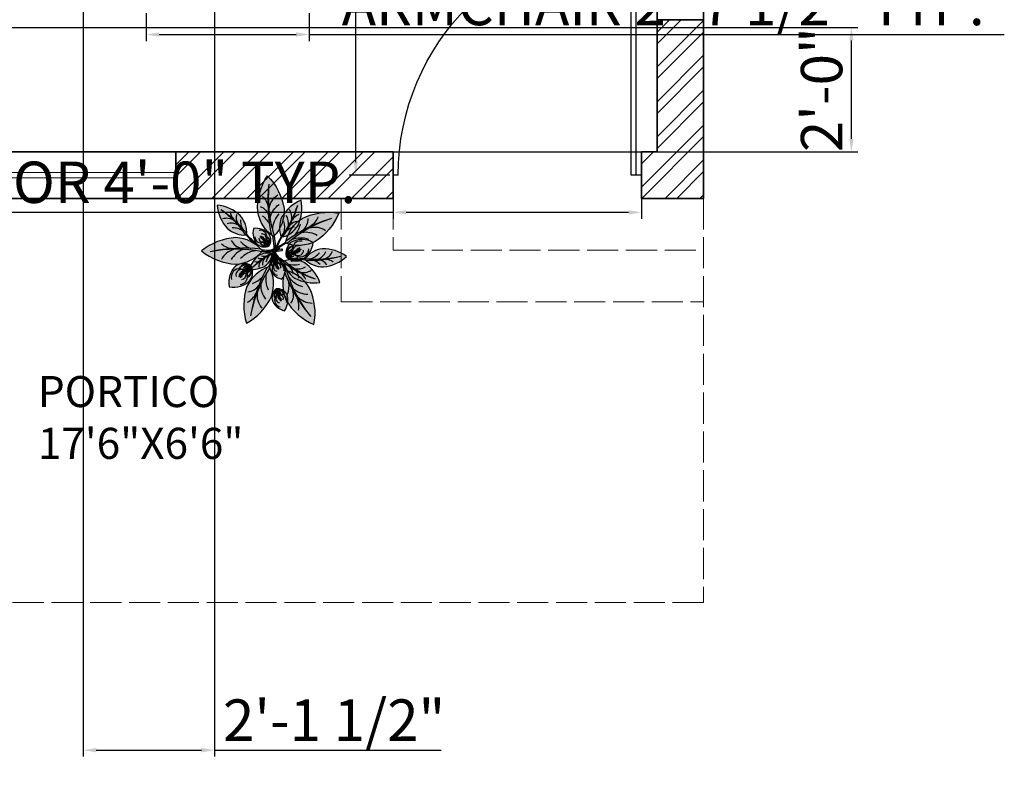
# Model space of a CAD drawing. Units: inches. Extents: x 3595 to 4516, y 2363 to 2965.
# Tile 8 of 12: x 4309 to 4499, y 2363 to 2512. Entities that reach past the tile are written whole.
import ezdxf

# ---------------------------------------------------------------- set-up
doc = ezdxf.new("R2010")
doc.units = ezdxf.units.IN
doc.linetypes.add('ACAD_ISO02W100', pattern=[15, 12, -3])
for name, color, linetype, lineweight in [('A-ANNO-DIMS', 2, 'Continuous', 18), ('A-AREA-IDEN', 7, 'Continuous', 18), ('A-DOOR', 4, 'Continuous', 25), ('A-FLOR-OTLN', 7, 'ACAD_ISO02W100', 18), ('A-FLOR-STRS-BYND', 7, 'ACAD_ISO02W100', 18), ('A-GLAZ', 4, 'Continuous', 18), ('A-WALL', 7, 'Continuous', 35), ('L-PLNT', 3, 'Continuous', 13)]:
    doc.layers.add(name, color=color, linetype=linetype, lineweight=lineweight)
doc.layers.add('A-WALL-PATT', color=251, linetype='Continuous', lineweight=13, true_color=0x636466)
doc.layers.add('MESA', color=7, linetype='Continuous')
doc.styles.get("Standard").update_dxf_attribs({"font": 'arial.ttf'})
doc.dimstyles.new('ISO-25', dxfattribs={"dimtxt": 8, "dimasz": 2.5, "dimexe": 1.25, "dimexo": 0.625, "dimtad": 1, "dimdec": 1, "dimlunit": 3, "dimtxsty": 'Standard', "dimcen": 2.5, "dimadec": 0, "dimazin": 0, "dimtfac": 1, "dimtdec": 1, "dimtmove": 0, "dimatfit": 3, "dimfxl": 1, "dimarcsym": 0})

# ---------------------------------------------------------------- blocks, each defined once
blk = doc.blocks.new('D')
for p, q in [((1, 0), (1, 46)), ((2, 0), (2, 46)), ((0, 0), (2, 0)), ((47, 0), (48, 0))]:
    blk.add_line(p, q)
at = {"ltscale": 0.5}
blk.add_arc((1, 0), 46, 0, 90, dxfattribs=at)
blk = doc.blocks.new('folha Ant')
at = {"layer": 'MESA', "ltscale": 0.8}
h = blk.add_hatch(color=256, dxfattribs=at)
h.dxf.hatch_style = 1
h.set_gradient(color1=(103, 159, 96), color2=(179, 207, 175), one_color=1, tint=0.75, name='INVCURVED')
h.paths.add_polyline_path([(0.2266, 0.0676, 0.199512), (0.0989, 0.0067, 0.09675), (0.3533, 0.0075, -0.086654), (0.1023, -0.0053, 0.192489), (0.2266, -0.0624, 0.158608), (0.3953, 0.0026, 0.158608)])
h = blk.add_hatch(color=256, dxfattribs=at)
h.dxf.hatch_style = 1
h.set_gradient(color1=(179, 116, 77), color2=(114, 74, 49), one_color=1, tint=0.32, name='CURVED')
h.paths.add_polyline_path([(0.05, -0.0003), (0.0485, 0.0057, 0.033108), (0, 0, 0.809082), (0.002, -0.006, -0.032777)])
h.paths.add_polyline_path([(0.0973, 0.0049, 0.033108), (0.0485, 0.0057), (0.05, -0.0003, -0.032777), (0.0983, -0.001), (0.0953, 0.0026)])
h = blk.add_hatch(color=256, dxfattribs=at)
h.dxf.hatch_style = 1
h.set_gradient(color1=(103, 159, 96), color2=(52, 80, 48), one_color=1, tint=0.25)
h.paths.add_polyline_path([(0.3533, 0.0075, -0.09675), (0.0989, 0.0067, 0.007527), (0.0953, 0.0026, 0.014292), (0.1023, -0.0053, 0.086654)])
blk.add_lwpolyline([(0.0983, -0.001), (0.0953, 0.0026), (0.0973, 0.0049, 0.066288), (0, 0, 0.809082), (0.002, -0.006, -0.065625)], format="xyb", close=True, dxfattribs=at)
for centre, radius, start, end in [((0.2359, -0.1164), 0.1842, 92.9121, 139.7695), ((0.211, -0.2242), 0.2922, 50.9055, 86.9554), ((0.2359, 0.1215), 0.1842, 220.2305, 267.0879), ((0.2242, 0.6583), 0.6635, 259.119, 281.2235), ((0.1912, 0.7199), 0.7306, 263.0097, 282.8199), ((0.1144, 0.1192), 0.1187, 277.6411, 318.482), ((0.1515, 0.1013), 0.1129, 290.5634, 330.4539), ((0.211, 0.2293), 0.2922, 273.0446, 309.0945), ((0.2123, 0.0879), 0.0955, 283.0013, 333.1911), ((0.1127, -0.1239), 0.1214, 41.7528, 70.1061), ((0.1853, -0.0821), 0.0727, 27.7376, 79.2347), ((0.2381, -0.0995), 0.0902, 48.8027, 88.011)]:
    blk.add_arc(centre, radius, start, end, dxfattribs=at)
blk = doc.blocks.new('folha A')
at = {"layer": 'MESA', "ltscale": 0.8}
h = blk.add_hatch(color=256, dxfattribs=at)
h.dxf.hatch_style = 1
h.set_gradient(color1=(237, 238, 238), one_color=1, tint=1)
h.paths.add_polyline_path([(0.15, 0, 0.256909), (0.0543, 0.05, 0.240303), (0.0028, 0.0075, -0.358381), (0.0489, 0.0306, 0.270233), (0, 0, -0.348977), (0.0363, 0.0149, 0.25095), (0.0039, 0, -0.245389), (0.0298, 0.008, 0.153246), (0.0082, 0, 0.15184), (0.0296, -0.008, 0.001374), (0.0298, -0.008, -0.245389), (0.0039, 0, 0.25095), (0.0363, -0.0149, -0.348977), (0, 0, 0.270233), (0.0489, -0.0306, -0.358381), (0.0028, -0.0075, 0.240303), (0.0543, -0.05, 0.256909)])
edge = h.paths.add_edge_path(flags=16)
edge.add_arc((0.0098, 0.0552), 0.0552, 269.916, 271.4154, ccw=False)
edge.add_arc((0.011, -0.0487), 0.0487, 89.8163, 91.5152, ccw=False)
edge.add_arc((0.0098, 0.0552), 0.0552, 271.4154, 288.9745)
edge.add_spline(control_points=[(0.0278, 0.003), (0.0281, 0.003), (0.03, 0.0028), (0.032, 0.0025), (0.0337, 0.0022)], knot_values=[0.247151, 0.247151, 0.247151, 0.247151, 0.247786, 0.253074, 0.253074, 0.253074, 0.253074], degree=3, periodic=0)
edge.add_spline(control_points=[(0.0337, 0.0022), (0.0349, 0.0021), (0.0361, 0.0019), (0.0372, 0.0017)], knot_values=[0.243636, 0.243636, 0.243636, 0.243636, 0.247151, 0.247151, 0.247151, 0.247151], degree=3, periodic=0)
edge.add_spline(control_points=[(0.0372, 0.0017), (0.0385, 0.0015), (0.0405, 0.0013), (0.0424, 0.0011), (0.0431, 0.0011)], knot_values=[0.23773, 0.23773, 0.23773, 0.23773, 0.241748, 0.243636, 0.243636, 0.243636, 0.243636], degree=3, periodic=0)
edge.add_spline(control_points=[(0.0431, 0.0011), (0.044, 0.001), (0.045, 0.001), (0.0459, 0.001)], knot_values=[0.234818, 0.234818, 0.234818, 0.234818, 0.23773, 0.23773, 0.23773, 0.23773], degree=3, periodic=0)
edge.add_spline(control_points=[(0.0459, 0.001), (0.0472, 0.0009), (0.0485, 0.0009), (0.0498, 0.0009)], knot_values=[0.230931, 0.230931, 0.230931, 0.230931, 0.234818, 0.234818, 0.234818, 0.234818], degree=3, periodic=0)
edge.add_spline(control_points=[(0.0498, 0.0009), (0.0513, 0.0009), (0.0528, 0.0009), (0.0543, 0.0009)], knot_values=[0.226471, 0.226471, 0.226471, 0.226471, 0.230931, 0.230931, 0.230931, 0.230931], degree=3, periodic=0)
edge.add_spline(control_points=[(0.0543, 0.0009), (0.0547, 0.0009), (0.0564, 0.001), (0.0581, 0.001), (0.0594, 0.0011)], knot_values=[0.221526, 0.221526, 0.221526, 0.221526, 0.222579, 0.226471, 0.226471, 0.226471, 0.226471], degree=3, periodic=0)
edge.add_spline(control_points=[(0.0594, 0.0011), (0.0609, 0.0012), (0.0623, 0.0014), (0.0637, 0.0017)], knot_values=[0.217168, 0.217168, 0.217168, 0.217168, 0.221526, 0.221526, 0.221526, 0.221526], degree=3, periodic=0)
edge.add_spline(control_points=[(0.0637, 0.0017), (0.0648, 0.002), (0.066, 0.0024), (0.0672, 0.0029), (0.0674, 0.003)], knot_values=[0.213164, 0.213164, 0.213164, 0.213164, 0.216463, 0.217168, 0.217168, 0.217168, 0.217168], degree=3, periodic=0)
edge.add_spline(control_points=[(0.0674, 0.003), (0.0685, 0.0035), (0.07, 0.0044), (0.0718, 0.0051), (0.0724, 0.0052)], knot_values=[0.207777, 0.207777, 0.207777, 0.207777, 0.211372, 0.213164, 0.213164, 0.213164, 0.213164], degree=3, periodic=0)
edge.add_spline(control_points=[(0.0724, 0.0052), (0.0729, 0.0053), (0.0744, 0.0054), (0.0757, 0.0044), (0.0762, 0.0036)], knot_values=[0.203445, 0.203445, 0.203445, 0.203445, 0.204995, 0.207777, 0.207777, 0.207777, 0.207777], degree=3, periodic=0)
edge.add_spline(control_points=[(0.0762, 0.0036), (0.0763, 0.0036), (0.0768, 0.0026), (0.0767, 0.0012), (0.0763, 0), (0.0763, -0.0001)], knot_values=[0.199694, 0.199694, 0.199694, 0.199694, 0.199863, 0.203137, 0.203445, 0.203445, 0.203445, 0.203445], degree=3, periodic=0)
edge.add_spline(control_points=[(0.0763, -0.0001), (0.0761, -0.0008), (0.0757, -0.0017), (0.075, -0.0024), (0.0748, -0.0026)], knot_values=[0.196756, 0.196756, 0.196756, 0.196756, 0.198903, 0.199694, 0.199694, 0.199694, 0.199694], degree=3, periodic=0)
edge.add_spline(control_points=[(0.0748, -0.0026), (0.0743, -0.0031), (0.0734, -0.0037), (0.0725, -0.0042), (0.0722, -0.0043)], knot_values=[0.193643, 0.193643, 0.193643, 0.193643, 0.195869, 0.196756, 0.196756, 0.196756, 0.196756], degree=3, periodic=0)
edge.add_spline(control_points=[(0.0722, -0.0043), (0.0708, -0.0049), (0.0694, -0.0052), (0.0678, -0.0054)], knot_values=[0.189135, 0.189135, 0.189135, 0.189135, 0.193643, 0.193643, 0.193643, 0.193643], degree=3, periodic=0)
edge.add_spline(control_points=[(0.0678, -0.0054), (0.0677, -0.0054), (0.0667, -0.0056), (0.0657, -0.0057), (0.0648, -0.0058)], knot_values=[0.186092, 0.186092, 0.186092, 0.186092, 0.186502, 0.189135, 0.189135, 0.189135, 0.189135], degree=3, periodic=0)
edge.add_spline(control_points=[(0.0648, -0.0058), (0.0635, -0.0059), (0.0621, -0.006), (0.0608, -0.0061)], knot_values=[0.182083, 0.182083, 0.182083, 0.182083, 0.186092, 0.186092, 0.186092, 0.186092], degree=3, periodic=0)
edge.add_spline(control_points=[(0.0608, -0.0061), (0.0596, -0.0062), (0.0584, -0.0062), (0.0571, -0.0062)], knot_values=[0.178391, 0.178391, 0.178391, 0.178391, 0.182083, 0.182083, 0.182083, 0.182083], degree=3, periodic=0)
edge.add_spline(control_points=[(0.0571, -0.0062), (0.0568, -0.0062), (0.0555, -0.0063), (0.0543, -0.0063), (0.0534, -0.0063)], knot_values=[0.17468, 0.17468, 0.17468, 0.17468, 0.175797, 0.178391, 0.178391, 0.178391, 0.178391], degree=3, periodic=0)
edge.add_spline(control_points=[(0.0534, -0.0063), (0.0525, -0.0063), (0.0516, -0.0063), (0.0506, -0.0063)], knot_values=[0.171864, 0.171864, 0.171864, 0.171864, 0.17468, 0.17468, 0.17468, 0.17468], degree=3, periodic=0)
edge.add_spline(control_points=[(0.0506, -0.0063), (0.0494, -0.0063), (0.0482, -0.0063), (0.047, -0.0062)], knot_values=[0.16826, 0.16826, 0.16826, 0.16826, 0.171864, 0.171864, 0.171864, 0.171864], degree=3, periodic=0)
edge.add_spline(control_points=[(0.047, -0.0062), (0.0453, -0.0061), (0.0434, -0.006), (0.0414, -0.0057), (0.0411, -0.0057)], knot_values=[0.162342, 0.162342, 0.162342, 0.162342, 0.167388, 0.16826, 0.16826, 0.16826, 0.16826], degree=3, periodic=0)
edge.add_spline(control_points=[(0.0411, -0.0057), (0.0399, -0.0055), (0.0386, -0.0053), (0.0374, -0.005)], knot_values=[0.158654, 0.158654, 0.158654, 0.158654, 0.162342, 0.162342, 0.162342, 0.162342], degree=3, periodic=0)
edge.add_spline(control_points=[(0.0374, -0.005), (0.0365, -0.0049), (0.0357, -0.0047), (0.0348, -0.0045)], knot_values=[0.156033, 0.156033, 0.156033, 0.156033, 0.158654, 0.158654, 0.158654, 0.158654], degree=3, periodic=0)
edge.add_spline(control_points=[(0.0348, -0.0045), (0.0335, -0.0043), (0.0317, -0.004), (0.03, -0.0037), (0.0295, -0.0036)], knot_values=[0.15048, 0.15048, 0.15048, 0.15048, 0.154549, 0.156033, 0.156033, 0.156033, 0.156033], degree=3, periodic=0)
edge.add_arc((0.011, -0.0487), 0.0487, 67.7054, 89.8163)
h = blk.add_hatch(color=256, dxfattribs=at)
h.dxf.hatch_style = 1
h.set_gradient(color1=(117, 211, 105), one_color=1, tint=1)
h.paths.add_polyline_path([(0.0489, 0.0306, 0.358381), (0.0028, 0.0075, 0.02724), (0, 0, -0.270233)])
h.paths.add_polyline_path([(0.0039, 0, -0.25095), (0.0363, 0.0149, 0.348977), (0, 0, 0.348977), (0.0363, -0.0149, -0.25095)])
h.paths.add_polyline_path([(0.0298, 0.008, 0.245389), (0.0039, 0, 0.245389), (0.0298, -0.008, -0.153246), (0.0082, 0, -0.153246)], flags=17)
h.paths.add_polyline_path([(0, 0, 0.02724), (0.0028, -0.0075, 0.358381), (0.0489, -0.0306, -0.270233)])
h = blk.add_hatch(color=256, dxfattribs=at)
h.dxf.hatch_style = 1
h.set_gradient(color1=(68, 182, 53), color2=(121, 213, 109), one_color=1, tint=0.63, name='CYLINDER')
edge = h.paths.add_edge_path()
edge.add_spline(control_points=[(0.0722, -0.0043), (0.0725, -0.0042), (0.0734, -0.0037), (0.0743, -0.0031), (0.0748, -0.0026)], knot_values=[0.193643, 0.193643, 0.193643, 0.193643, 0.194531, 0.196756, 0.196756, 0.196756, 0.196756], degree=3, periodic=0)
edge.add_spline(control_points=[(0.0748, -0.0026), (0.075, -0.0024), (0.0757, -0.0017), (0.0761, -0.0008), (0.0763, -0.0001)], knot_values=[0.196756, 0.196756, 0.196756, 0.196756, 0.197548, 0.199694, 0.199694, 0.199694, 0.199694], degree=3, periodic=0)
edge.add_spline(control_points=[(0.0763, -0.0001), (0.0763, 0), (0.0767, 0.0012), (0.0768, 0.0026), (0.0763, 0.0036), (0.0762, 0.0036)], knot_values=[0.199694, 0.199694, 0.199694, 0.199694, 0.200002, 0.203276, 0.203445, 0.203445, 0.203445, 0.203445], degree=3, periodic=0)
edge.add_spline(control_points=[(0.0762, 0.0036), (0.0757, 0.0044), (0.0744, 0.0054), (0.0729, 0.0053), (0.0724, 0.0052)], knot_values=[0.203445, 0.203445, 0.203445, 0.203445, 0.206228, 0.207777, 0.207777, 0.207777, 0.207777], degree=3, periodic=0)
edge.add_spline(control_points=[(0.0724, 0.0052), (0.0718, 0.0051), (0.07, 0.0044), (0.0685, 0.0035), (0.0674, 0.003)], knot_values=[0.207777, 0.207777, 0.207777, 0.207777, 0.20957, 0.213164, 0.213164, 0.213164, 0.213164], degree=3, periodic=0)
edge.add_spline(control_points=[(0.0674, 0.003), (0.0672, 0.0029), (0.066, 0.0024), (0.0648, 0.002), (0.0637, 0.0017)], knot_values=[0.213164, 0.213164, 0.213164, 0.213164, 0.213868, 0.217168, 0.217168, 0.217168, 0.217168], degree=3, periodic=0)
edge.add_spline(control_points=[(0.0637, 0.0017), (0.0623, 0.0014), (0.0609, 0.0012), (0.0594, 0.0011)], knot_values=[0.217168, 0.217168, 0.217168, 0.217168, 0.221526, 0.221526, 0.221526, 0.221526], degree=3, periodic=0)
edge.add_spline(control_points=[(0.0594, 0.0011), (0.0581, 0.001), (0.0564, 0.001), (0.0547, 0.0009), (0.0543, 0.0009)], knot_values=[0.221526, 0.221526, 0.221526, 0.221526, 0.225418, 0.226471, 0.226471, 0.226471, 0.226471], degree=3, periodic=0)
edge.add_spline(control_points=[(0.0543, 0.0009), (0.0528, 0.0009), (0.0513, 0.0009), (0.0498, 0.0009)], knot_values=[0.226471, 0.226471, 0.226471, 0.226471, 0.230931, 0.230931, 0.230931, 0.230931], degree=3, periodic=0)
edge.add_spline(control_points=[(0.0498, 0.0009), (0.0485, 0.0009), (0.0472, 0.0009), (0.0459, 0.001)], knot_values=[0.230931, 0.230931, 0.230931, 0.230931, 0.234818, 0.234818, 0.234818, 0.234818], degree=3, periodic=0)
edge.add_spline(control_points=[(0.0459, 0.001), (0.045, 0.001), (0.044, 0.001), (0.0431, 0.0011)], knot_values=[0.234818, 0.234818, 0.234818, 0.234818, 0.23773, 0.23773, 0.23773, 0.23773], degree=3, periodic=0)
edge.add_spline(control_points=[(0.0431, 0.0011), (0.0424, 0.0011), (0.0405, 0.0013), (0.0385, 0.0015), (0.0372, 0.0017)], knot_values=[0.23773, 0.23773, 0.23773, 0.23773, 0.239619, 0.243636, 0.243636, 0.243636, 0.243636], degree=3, periodic=0)
edge.add_spline(control_points=[(0.0372, 0.0017), (0.0361, 0.0019), (0.0349, 0.0021), (0.0337, 0.0022)], knot_values=[0.243636, 0.243636, 0.243636, 0.243636, 0.247151, 0.247151, 0.247151, 0.247151], degree=3, periodic=0)
edge.add_spline(control_points=[(0.0337, 0.0022), (0.032, 0.0025), (0.03, 0.0028), (0.0281, 0.003), (0.0278, 0.003)], knot_values=[0.247151, 0.247151, 0.247151, 0.247151, 0.25244, 0.253074, 0.253074, 0.253074, 0.253074], degree=3, periodic=0)
edge.add_arc((0.011, 0.0487), 0.0487, 271.5152, 290.2274, ccw=False)
edge.add_arc((0.011, -0.0487), 0.0487, 67.7054, 88.4848, ccw=False)
edge.add_spline(control_points=[(0.0295, -0.0036), (0.03, -0.0037), (0.0317, -0.004), (0.0335, -0.0043), (0.0348, -0.0045)], knot_values=[0.15048, 0.15048, 0.15048, 0.15048, 0.151964, 0.156033, 0.156033, 0.156033, 0.156033], degree=3, periodic=0)
edge.add_spline(control_points=[(0.0348, -0.0045), (0.0357, -0.0047), (0.0365, -0.0049), (0.0374, -0.005)], knot_values=[0.156033, 0.156033, 0.156033, 0.156033, 0.158654, 0.158654, 0.158654, 0.158654], degree=3, periodic=0)
edge.add_spline(control_points=[(0.0374, -0.005), (0.0386, -0.0053), (0.0399, -0.0055), (0.0411, -0.0057)], knot_values=[0.158654, 0.158654, 0.158654, 0.158654, 0.162342, 0.162342, 0.162342, 0.162342], degree=3, periodic=0)
edge.add_spline(control_points=[(0.0411, -0.0057), (0.0414, -0.0057), (0.0434, -0.006), (0.0453, -0.0061), (0.047, -0.0062)], knot_values=[0.162342, 0.162342, 0.162342, 0.162342, 0.163214, 0.16826, 0.16826, 0.16826, 0.16826], degree=3, periodic=0)
edge.add_spline(control_points=[(0.047, -0.0062), (0.0482, -0.0063), (0.0494, -0.0063), (0.0506, -0.0063)], knot_values=[0.16826, 0.16826, 0.16826, 0.16826, 0.171864, 0.171864, 0.171864, 0.171864], degree=3, periodic=0)
edge.add_spline(control_points=[(0.0506, -0.0063), (0.0516, -0.0063), (0.0525, -0.0063), (0.0534, -0.0063)], knot_values=[0.171864, 0.171864, 0.171864, 0.171864, 0.17468, 0.17468, 0.17468, 0.17468], degree=3, periodic=0)
edge.add_spline(control_points=[(0.0534, -0.0063), (0.0543, -0.0063), (0.0555, -0.0063), (0.0568, -0.0062), (0.0571, -0.0062)], knot_values=[0.17468, 0.17468, 0.17468, 0.17468, 0.177274, 0.178391, 0.178391, 0.178391, 0.178391], degree=3, periodic=0)
edge.add_spline(control_points=[(0.0571, -0.0062), (0.0584, -0.0062), (0.0596, -0.0062), (0.0608, -0.0061)], knot_values=[0.178391, 0.178391, 0.178391, 0.178391, 0.182083, 0.182083, 0.182083, 0.182083], degree=3, periodic=0)
edge.add_spline(control_points=[(0.0608, -0.0061), (0.0621, -0.006), (0.0635, -0.0059), (0.0648, -0.0058)], knot_values=[0.182083, 0.182083, 0.182083, 0.182083, 0.186092, 0.186092, 0.186092, 0.186092], degree=3, periodic=0)
edge.add_spline(control_points=[(0.0648, -0.0058), (0.0657, -0.0057), (0.0667, -0.0056), (0.0677, -0.0054), (0.0678, -0.0054)], knot_values=[0.186092, 0.186092, 0.186092, 0.186092, 0.188726, 0.189135, 0.189135, 0.189135, 0.189135], degree=3, periodic=0)
edge.add_spline(control_points=[(0.0678, -0.0054), (0.0694, -0.0052), (0.0708, -0.0049), (0.0722, -0.0043)], knot_values=[0.189135, 0.189135, 0.189135, 0.189135, 0.193643, 0.193643, 0.193643, 0.193643], degree=3, periodic=0)
for p, q in [((0.0299, -0.0008), (0.0236, 0.0003)), ((0.0324, 0.0004), (0.0358, 0.0051)), ((0.0367, 0.001), (0.0414, 0.0073)), ((0.0435, -0.0027), (0.0427, 0.0041)), ((0.0455, -0.0007), (0.0466, 0.0032)), ((0.0507, -0.0021), (0.0477, 0.0086)), ((0.0545, -0.0006), (0.0538, 0.005)), ((0.0604, -0.0013), (0.0571, 0.0065)), ((0.0637, -0.0003), (0.0638, 0.0057)), ((0.0674, 0.0003), (0.0674, 0.0088)), ((0.071, 0.0011), (0.0736, 0.0087)), ((0.0744, 0.0005), (0.0836, -0.0024)), ((0.0745, 0.0023), (0.0809, 0.0072)), ((0.0331, -0.0017), (0.0356, -0.0058)), ((0.0359, -0.0021), (0.0384, -0.0071)), ((0.04, -0.0018), (0.0423, -0.0098)), ((0.0474, -0.0047), (0.0459, -0.0105)), ((0.0512, -0.005), (0.0493, -0.009)), ((0.0546, -0.0037), (0.0519, -0.0097)), ((0.0571, -0.0045), (0.0573, -0.0126)), ((0.0629, -0.0036), (0.0579, -0.0096)), ((0.0649, -0.0044), (0.0646, -0.0097)), ((0.0679, -0.003), (0.0676, -0.0121)), ((0.0718, -0.0029), (0.0733, -0.0082)), ((0.0731, -0.0013), (0.0781, -0.005))]:
    blk.add_line(p, q, dxfattribs=at)
for centre, radius, start, end in [((0.0702, -0.0218), 0.0735, 102.4876, 162.7777), ((0.0567, -0.062), 0.112, 33.595, 91.2278), ((0.0507, -0.0267), 0.0573, 91.7664, 152.2545), ((0.0275, -0.0154), 0.0315, 73.8983, 150.8496), ((0.0399, -0.009), 0.0406, 77.1426, 158.365), ((0.034, -0.0228), 0.0378, 86.5852, 142.9351), ((0.0245, -0.0208), 0.0293, 79.5747, 134.724), ((0.0317, -0.0305), 0.0385, 92.8652, 127.7155), ((0.0067, 0.0482), 0.0483, 273.5313, 328.711), ((0.0098, 0.0552), 0.0552, 269.916, 311.5613), ((0.011, -0.0487), 0.0487, 43.3703, 91.5152), ((0.0655, -0.0023), 0.025, 51.9712, 139.685), ((0.0788, 0.0012), 0.0378, 48.9446, 144.5333), ((0.0507, 0.0267), 0.0573, 207.7455, 268.2336), ((0.0275, 0.0154), 0.0315, 209.1504, 286.1017), ((0.0702, 0.0218), 0.0735, 197.2223, 257.5124), ((0.0399, 0.009), 0.0406, 201.635, 282.8574), ((0.034, 0.0228), 0.0378, 217.0649, 273.4148), ((0.0245, 0.0208), 0.0293, 225.276, 280.4253), ((0.0317, 0.0305), 0.0385, 232.2845, 267.1348), ((0.0067, -0.0482), 0.0483, 31.289, 86.4687), ((0.0676, -0.0011), 0.0254, 213.677, 332.8415), ((0.0804, 0.0017), 0.0409, 217.4348, 331.7322), ((0.0567, 0.062), 0.112, 268.7722, 326.405)]:
    blk.add_arc(centre, radius, start, end, dxfattribs=at)
blk.add_open_spline([(0.0295, -0.0036), (0.03, -0.0037), (0.0339, -0.0043), (0.0429, -0.0064), (0.0552, -0.0064), (0.0655, -0.0059), (0.0723, -0.0047), (0.0754, -0.0023), (0.0766, 0.0004), (0.0769, 0.0036), (0.0738, 0.0058), (0.0702, 0.0046), (0.0648, 0.0013), (0.0544, 0.0009), (0.0416, 0.0008), (0.0325, 0.0025), (0.0281, 0.003), (0.0278, 0.003)], degree=3, knots=[0.1504802, 0.1504802, 0.1504802, 0.1504802, 0.1519644, 0.163214, 0.177274, 0.1887256, 0.1945307, 0.1975476, 0.2000024, 0.2032763, 0.2062279, 0.2095699, 0.2138685, 0.2254176, 0.2396186, 0.2524399, 0.2530743, 0.2530743, 0.2530743, 0.2530743], dxfattribs=at)
blk = doc.blocks.new('Anturio Completa')
at = {"layer": 'MESA', "xscale": -1}
for p, rotation in [((0.0382, -0.3934), 275.9103487005753), ((0.0047, -0.3743), 209.3422747969654)]:
    blk.add_blockref('folha Ant', p, dxfattribs=dict(at, rotation=rotation))
at = {"layer": 'MESA'}
for name, p, xscale, yscale, zscale, rotation in [('folha Ant', (-0.0545, -0.3355), 0.6875195991113106, 0.6875195991113106, 0.6875195991113106, 134.6123703789177), ('folha Ant', (0.0396, -0.3604), 0.6875195991112988, 0.6875195991112988, 0.6875195991112988, 62.02852832027476), ('folha A', (0.0091, -0.3436), 0.7678141644548924, 0.7678141644548924, 0.7678141644548924, 132.2423739965673), ('folha Ant', (0.06, -0.3566), 0.4588451896756128, 0.4588451896756128, 0.4588451896756128, 214.0760858842101), ('folha A', (0.0322, -0.3992), 0.7678141644548587, 0.7678141644548587, 0.7678141644548587, 290.0444626994612), ('folha Ant', (0.0225, -0.3869), 0.6875195991113232, 0.6875195991113232, 0.6875195991113232, 329.7037252995857), ('folha Ant', (0.1178, -0.4144), 0.6875195991112375, 0.6875195991112375, 0.6875195991112375, 3.732606609119443), ('folha A', (0.0446, -0.5537), 0.7678141644548587, 0.7678141644548587, 0.7678141644548587, 290.0444626994612)]:
    blk.add_blockref(name, p, dxfattribs=dict(at, xscale=xscale, yscale=yscale, zscale=zscale, rotation=rotation))
for name, p, rotation in [('folha A', (0.0917, -0.3951), 27.20904127110871), ('folha Ant', (0.0722, -0.3656), 180), ('folha Ant', (0.0428, -0.3558), 248.0349850699403), ('folha Ant', (0.0423, -0.3813), 297.7195320534174), ('folha A', (-0.0806, -0.4387), 224.8255080541778)]:
    blk.add_blockref(name, p, dxfattribs=dict(at, rotation=rotation))
blk = doc.blocks.new('WIN-GLAZING-66IN')
for p, q in [((0, 1), (66, 1)), ((0, 0), (66, 0))]:
    blk.add_line(p, q)
blk = doc.blocks.new('PORTICO-ENTRY-STEPS')
at = {"ltscale": 0.5}
for p, q in [((0, 20), (0, 0)), ((10, 20), (10, 10)), ((10, 10), (70, 10)), ((0, 0), (70, 0))]:
    blk.add_line(p, q, dxfattribs=at)
blk = doc.blocks.new('*D113')
at = {"layer": 'A-ANNO-DIMS', "color": 0, "lineweight": -2, "transparency": 16777216}
for p, q in [((4381.24, 2480.92), (4381.24, 2473.09)), ((4429.24, 2480.92), (4429.24, 2473.09)), ((4381.24, 2474.34), (4251.53, 2474.34)), ((4426.74, 2474.34), (4383.74, 2474.34))]:
    blk.add_line(p, q, dxfattribs=at)
at = {"layer": 'A-ANNO-DIMS', "color": 0, "transparency": 16777216}
for points in [[(4383.74, 2474.76), (4383.74, 2473.93), (4381.24, 2474.34)], [(4426.74, 2474.76), (4426.74, 2473.93), (4429.24, 2474.34)]]:
    blk.add_solid(points, dxfattribs=at)
at = {"layer": 'Defpoints', "color": 0, "transparency": 16777216}
for p in [(4381.24, 2481.54), (4429.24, 2481.54), (4381.24, 2474.34)]:
    blk.add_point(p, dxfattribs=at)
at = {"layer": 'A-ANNO-DIMS', "color": 0, "transparency": 16777216, "insert": (4315.14, 2479.11), "char_height": 8, "attachment_point": 5}
blk.add_mtext('ENTRY DOOR 4\'-0" TYP.', dxfattribs=at)
blk = doc.blocks.new('*D114')
at = {"layer": 'A-ANNO-DIMS', "color": 0, "lineweight": -2, "transparency": 16777216}
for p, q in [((4374.04, 2527.54), (4374.04, 2586.27)), ((4380.62, 2527.54), (4372.79, 2527.54)), ((4374.04, 2484.04), (4374.04, 2525.04)), ((4380.62, 2481.54), (4372.79, 2481.54))]:
    blk.add_line(p, q, dxfattribs=at)
at = {"layer": 'A-ANNO-DIMS', "color": 0, "transparency": 16777216}
for points in [[(4373.63, 2525.04), (4374.46, 2525.04), (4374.04, 2527.54)], [(4373.63, 2484.04), (4374.46, 2484.04), (4374.04, 2481.54)]]:
    blk.add_solid(points, dxfattribs=at)
at = {"layer": 'Defpoints', "color": 0, "transparency": 16777216}
for p in [(4374.04, 2527.54), (4381.24, 2527.54), (4381.24, 2481.54)]:
    blk.add_point(p, dxfattribs=at)
at = {"layer": 'A-ANNO-DIMS', "color": 0, "transparency": 16777216, "insert": (4369.33, 2558.16), "char_height": 8, "attachment_point": 5, "rotation": 90}
blk.add_mtext('3\'-10" TYP.', dxfattribs=at)
blk = doc.blocks.new('*D139')
at = {"layer": 'A-ANNO-DIMS', "color": 0, "lineweight": -2, "transparency": 16777216}
for p, q in [((4333.52, 2512.78), (4333.52, 2507.43)), ((4365.01, 2512.78), (4365.01, 2507.43)), ((4336.02, 2508.68), (4362.51, 2508.68)), ((4365.01, 2508.68), (4499.34, 2508.68))]:
    blk.add_line(p, q, dxfattribs=at)
at = {"layer": 'A-ANNO-DIMS', "color": 0, "transparency": 16777216}
for points in [[(4336.02, 2509.1), (4336.02, 2508.27), (4333.52, 2508.68)], [(4362.51, 2509.1), (4362.51, 2508.27), (4365.01, 2508.68)]]:
    blk.add_solid(points, dxfattribs=at)
at = {"layer": 'Defpoints', "color": 0, "transparency": 16777216}
for p in [(4333.52, 2513.41), (4365.01, 2513.41), (4365.01, 2508.68)]:
    blk.add_point(p, dxfattribs=at)
at = {"layer": 'A-ANNO-DIMS', "color": 0, "transparency": 16777216, "insert": (4433.43, 2513.44), "char_height": 8, "attachment_point": 5}
blk.add_mtext('ARMCHAIR 2\'-7 1/2" TYP.', dxfattribs=at)
blk = doc.blocks.new('*D160')
at = {"layer": 'A-ANNO-DIMS', "color": 0, "lineweight": -2, "transparency": 16777216}
for p, q in [((4114.87, 2510.04), (4471.04, 2510.04)), ((4469.79, 2488.54), (4469.79, 2507.54)), ((4090.87, 2486.04), (4471.04, 2486.04))]:
    blk.add_line(p, q, dxfattribs=at)
at = {"layer": 'A-ANNO-DIMS', "color": 0, "transparency": 16777216}
for points in [[(4469.38, 2507.54), (4470.21, 2507.54), (4469.79, 2510.04)], [(4469.38, 2488.54), (4470.21, 2488.54), (4469.79, 2486.04)]]:
    blk.add_solid(points, dxfattribs=at)
at = {"layer": 'Defpoints', "color": 0, "transparency": 16777216}
for p in [(4114.24, 2510.04), (4469.79, 2510.04), (4090.24, 2486.04)]:
    blk.add_point(p, dxfattribs=at)
at = {"layer": 'A-ANNO-DIMS', "color": 0, "transparency": 16777216, "insert": (4465.08, 2498.04), "char_height": 8, "attachment_point": 5, "rotation": 90}
blk.add_mtext('2\'-0"', dxfattribs=at)
blk = doc.blocks.new('*D161')
at = {"layer": 'A-ANNO-DIMS', "color": 0, "lineweight": -2, "transparency": 16777216}
for p, q in [((4321.38, 2565.12), (4321.38, 2369.24)), ((4346.72, 2565.12), (4346.72, 2369.24)), ((4323.88, 2370.49), (4344.22, 2370.49)), ((4346.72, 2370.49), (4390.51, 2370.49))]:
    blk.add_line(p, q, dxfattribs=at)
at = {"layer": 'A-ANNO-DIMS', "color": 0, "transparency": 16777216}
for points in [[(4323.88, 2370.91), (4323.88, 2370.08), (4321.38, 2370.49)], [(4344.22, 2370.91), (4344.22, 2370.08), (4346.72, 2370.49)]]:
    blk.add_solid(points, dxfattribs=at)
at = {"layer": 'Defpoints', "color": 0, "transparency": 16777216}
for p in [(4321.38, 2565.75), (4346.72, 2565.75), (4346.72, 2370.49)]:
    blk.add_point(p, dxfattribs=at)
at = {"layer": 'A-ANNO-DIMS', "color": 0, "transparency": 16777216, "insert": (4369.86, 2375.26), "char_height": 8, "attachment_point": 5}
blk.add_mtext('2\'-1 1/2"', dxfattribs=at)

msp = doc.modelspace()

# ---------------------------------------------------------------- hatches: boundary and pattern name
at = {"layer": 'A-WALL-PATT'}
h = msp.add_hatch(dxfattribs=at)
h.set_pattern_fill('ANSI32', color=256, scale=0.5)
h.set_pattern_definition([(45, (441.351, 0), (-3.367596, 3.367596), []), (45, (443.596, 0), (-3.367596, 3.367596), [])])
h.paths.add_polyline_path([(4081.24, 2756.04), (4090.24, 2756.04), (4090.24, 2894.04), (4168.24, 2894.04), (4168.24, 2903.04), (4081.24, 2903.04)])
h.paths.add_polyline_path([(4216.24, 2903.04), (4216.24, 2894.04), (4222.24, 2894.04), (4222.24, 2792.04), (4231.24, 2792.04), (4231.24, 2894.04), (4241.74, 2894.04), (4241.74, 2903.04)])
h.paths.add_polyline_path([(4324.24, 2894.04), (4324.24, 2903.04), (4277.74, 2903.04), (4277.74, 2894.04), (4288.24, 2894.04), (4288.24, 2798.04), (4261.24, 2798.04), (4261.24, 2792.04), (4288.24, 2792.04), (4288.24, 2756.04), (4222.24, 2756.04), (4222.24, 2702.04), (4219.24, 2702.04), (4219.24, 2693.04), (4241.74, 2693.04), (4241.74, 2702.04), (4231.24, 2702.04), (4231.24, 2750.04), (4288.24, 2750.04), (4288.24, 2702.04), (4277.74, 2702.04), (4277.74, 2693.04), (4393.24, 2693.04), (4393.24, 2702.04), (4294.24, 2702.04), (4294.24, 2840.04), (4396.24, 2840.04), (4396.24, 2846.04), (4294.24, 2846.04), (4294.24, 2894.04)])
h.paths.add_polyline_path([(4390.24, 2894.04), (4390.24, 2876.04), (4396.24, 2876.04), (4396.24, 2894.04), (4432.24, 2894.04), (4432.24, 2795.04), (4441.24, 2795.04), (4441.24, 2903.04), (4360.24, 2903.04), (4360.24, 2894.04)])
h.paths.add_polyline_path([(4090.24, 2693.04), (4183.24, 2693.04), (4183.24, 2702.04), (4090.24, 2702.04), (4090.24, 2708.04), (4081.24, 2708.04), (4081.24, 2673.54), (4090.24, 2673.54)])
h.paths.add_polyline_path([(4090.24, 2600.04), (4183.24, 2600.04), (4183.24, 2606.04), (4090.24, 2606.04), (4090.24, 2625.54), (4081.24, 2625.54), (4081.24, 2561.04), (4090.24, 2561.04)])
h.paths.add_polyline_path([(4081.24, 2399.04), (4231.24, 2399.04), (4231.24, 2405.04), (4090.24, 2405.04), (4090.24, 2477.04), (4180.24, 2477.04), (4180.24, 2486.04), (4090.24, 2486.04), (4090.24, 2525.04), (4081.24, 2525.04)])
h.paths.add_polyline_path([(4231.24, 2486.04), (4231.24, 2606.04), (4219.24, 2606.04), (4219.24, 2600.04), (4222.24, 2600.04), (4222.24, 2486.04), (4216.24, 2486.04), (4216.24, 2477.04), (4273.24, 2477.04), (4273.24, 2486.04)])
h.paths.add_polyline_path([(4339.24, 2486.04), (4339.24, 2477.04), (4381.24, 2477.04), (4381.24, 2486.04)])
h.paths.add_polyline_path([(4432.24, 2486.04), (4429.24, 2486.04), (4429.24, 2477.04), (4441.24, 2477.04), (4441.24, 2511.54), (4432.24, 2511.54)])
h.paths.add_polyline_path([(4432.24, 2571.54), (4441.24, 2571.54), (4441.24, 2607.54), (4432.24, 2607.54)])
h.paths.add_polyline_path([(4441.24, 2747.04), (4432.24, 2747.04), (4432.24, 2702.04), (4429.24, 2702.04), (4429.24, 2693.04), (4432.24, 2693.04), (4432.24, 2667.54), (4441.24, 2667.54)])

# ---------------------------------------------------------------- linework, layer by layer
at = {"layer": 'A-FLOR-OTLN', "ltscale": 0.5}
for p, q in [((4441.24, 2477.04), (4441.24, 2399.04)), ((4441.24, 2399.04), (4231.24, 2399.04))]:
    msp.add_line(p, q, dxfattribs=at)
at = {"layer": 'A-WALL'}
for p, q in [((4432.24, 2693.04), (4432.24, 2486.04)), ((4441.24, 2511.54), (4432.24, 2511.54)), ((4231.24, 2486.04), (4381.24, 2486.04)), ((4339.24, 2486.04), (4339.24, 2477.04)), ((4381.24, 2486.04), (4381.24, 2477.04)), ((4429.24, 2486.04), (4432.24, 2486.04)), ((4429.24, 2486.04), (4429.24, 2477.04)), ((4090.24, 2477.04), (4381.24, 2477.04)), ((4429.24, 2477.04), (4441.24, 2477.04))]:
    msp.add_line(p, q, dxfattribs=at)
msp.add_lwpolyline([(4231.24, 2399.04), (4081.24, 2399.04), (4081.24, 2903.04), (4441.24, 2903.04), (4441.24, 2477.04)], dxfattribs=at)

# ---------------------------------------------------------------- block references
at = {"layer": 'A-DOOR', "xscale": -1}
msp.add_blockref('D', (4429.24, 2481.54), dxfattribs=at)
at = {"layer": 'A-FLOR-STRS-BYND'}
msp.add_blockref('PORTICO-ENTRY-STEPS', (4371.24, 2457.04), dxfattribs=at)
at = {"layer": 'A-GLAZ'}
msp.add_blockref('WIN-GLAZING-66IN', (4273.24, 2481.04), dxfattribs=at)
at = {"layer": 'L-PLNT', "xscale": 39.3701, "yscale": 39.3701, "zscale": 39.3701}
msp.add_blockref('Anturio Completa', (4356.95, 2481.4), dxfattribs=at)

# ---------------------------------------------------------------- texts
at = {"layer": 'A-AREA-IDEN', "insert": (4312.61, 2442.74), "char_height": 6, "attachment_point": 1}
msp.add_mtext_dynamic_manual_height_columns('{\\fTimes New Roman|b0|i0|c0|p18;PORTICO\\P17\'6"X6\'6"}', width=67.3508, gutter_width=12.5, heights=[0], dxfattribs=at)

# ---------------------------------------------------------------- dimensions: what is measured, and where the dimension line sits
at = {"layer": 'A-ANNO-DIMS'}
for base, p1, p2, angle, text, picture, middle in [((4374.04, 2527.54), (4381.24, 2481.54), (4381.24, 2527.54), 90, '<> TYP.', '*D114', (4369.33, 2558.16)), ((4381.24, 2474.34), (4429.24, 2481.54), (4381.24, 2481.54), 180, 'ENTRY DOOR <> TYP.', '*D113', (4315.14, 2479.11))]:
    dim = msp.add_linear_dim(base=base, p1=p1, p2=p2, angle=angle, text=text, dimstyle='ISO-25', override={"dimdec": 1, "dimlfac": 1, "dimrnd": 0, "dimzin": 1, "dimdsep": 46, "dimlunit": 4, "dimfrac": 2}, dxfattribs=at)
    dim.commit()
    dim.dimension.update_dxf_attribs({"geometry": picture, "text_midpoint": middle})
dim = msp.add_linear_dim(base=(4346.72, 2370.49), p1=(4321.38, 2565.75), p2=(4346.72, 2565.75), dimstyle='ISO-25', override={"dimdec": 1, "dimlfac": 1, "dimrnd": 0, "dimzin": 1, "dimdsep": 46, "dimlunit": 4, "dimfrac": 2}, dxfattribs=at)
dim.commit()
dim.dimension.update_dxf_attribs({"geometry": '*D161', "text_midpoint": (4369.86, 2375.26)})
dim = msp.add_linear_dim(base=(4365.01, 2508.68), p1=(4333.52, 2513.41), p2=(4365.01, 2513.41), text='ARMCHAIR <> TYP.', dimstyle='ISO-25', override={"dimdec": 1, "dimlfac": 1, "dimrnd": 0, "dimzin": 1, "dimdsep": 46, "dimlunit": 4, "dimfrac": 2}, dxfattribs=at)
dim.commit()
dim.dimension.update_dxf_attribs({"geometry": '*D139', "text_midpoint": (4433.43, 2513.44)})
dim = msp.add_linear_dim(base=(4469.79, 2510.04), p1=(4090.24, 2486.04), p2=(4114.24, 2510.04), angle=90, dimstyle='ISO-25', override={"dimdec": 1, "dimlfac": 1, "dimrnd": 0, "dimzin": 1, "dimdsep": 46, "dimlunit": 4, "dimfrac": 2}, dxfattribs=at)
dim.commit()
dim.dimension.update_dxf_attribs({"geometry": '*D160', "text_midpoint": (4465.08, 2498.04)})

doc.saveas('drawing.dxf')
